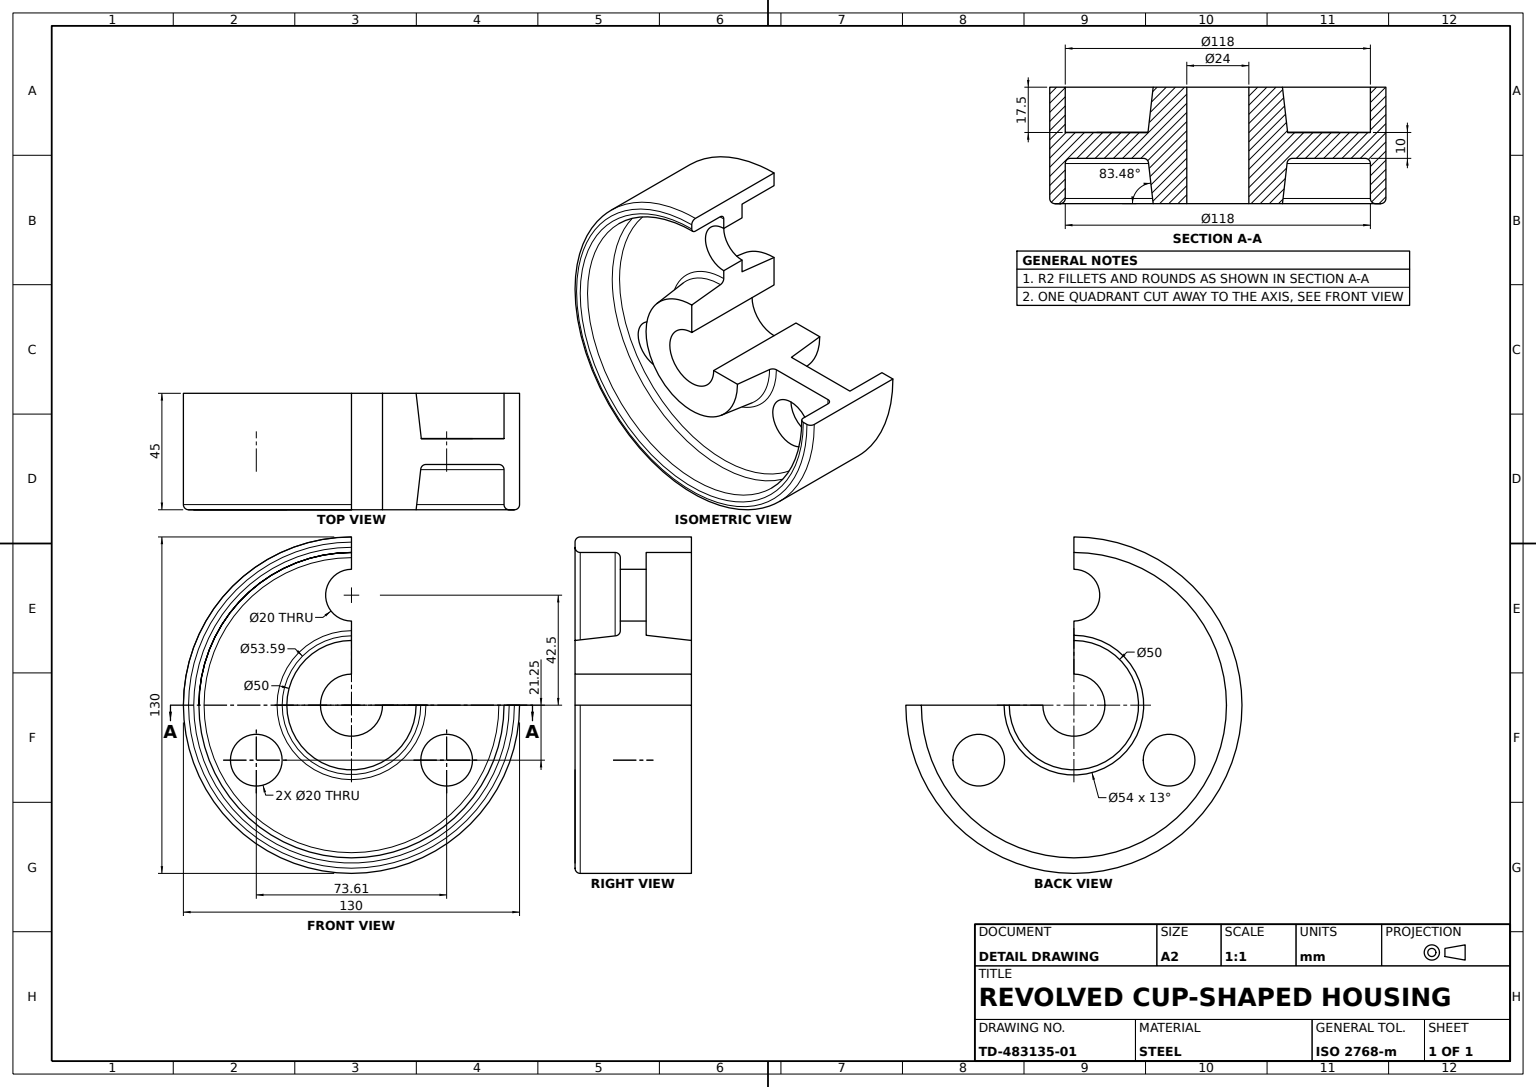
from build123d import *

# Parameters (mm, degrees)
RIM_SLOT_SKETCH_R         = 10
RIM_SLOT_CUT_DEPTH        = 96.949205312
EDGE_FILLET_R2_A_R        = 2
EDGE_FILLET_R2_B_R        = 2
WEB_RELIEF_CUT_DEPTH      = 96.94920538
WEB_RELIEF_CUT_DEPTH_BACK = 96.94920538


with BuildPart() as part:
    # Wheel Profile Sketch → Wheel Body Revolve (revolve)
    with BuildSketch(Plane.XY, mode=Mode.PRIVATE) as wheel_body_revolve_sk:
        Polygon((22.5, 12), (-22.5, 12), (-22.5, 25), (-5, 27), (-5, 59), (-22.5, 59), (-22.5, 65), (22.5, 65), (22.5, 59), (5, 59), (5, 27), (22.5, 25), align=None)
    revolve(wheel_body_revolve_sk.sketch.rotate(Axis((-53.084730572, 0, 0), (1, 0, 0)), 90), axis=Axis((-53.084730572, 0, 0), (1, 0, 0)))

    # Rim Slot Sketch → Rim Slot Cut (cut, through all)
    with BuildSketch(Plane(origin=(5, 0, 0), x_dir=(0, 0, -1), z_dir=(1, 0, 0))):
        with Locations((0, 42.5)):
            Circle(RIM_SLOT_SKETCH_R)
        with Locations((36.806079661, -21.25)):
            Circle(RIM_SLOT_SKETCH_R)
        with Locations((-36.806079661, -21.25)):
            Circle(RIM_SLOT_SKETCH_R)
    extrude(amount=-RIM_SLOT_CUT_DEPTH, mode=Mode.SUBTRACT)

    # Edge Fillet R2 A
    edge_fillet_r2_a_edges = [part.edges().sort_by_distance(p)[0] for p in [
        (22.5, 0, -65),
        (5, 0, -59),
        (5, 0, -27),
    ]]
    fillet(edge_fillet_r2_a_edges, radius=EDGE_FILLET_R2_A_R)

    # Edge Fillet R2 B
    edge_fillet_r2_b_edges = [part.edges().sort_by_distance(p)[0] for p in [
        (22.5, 0, -59),
    ]]
    fillet(edge_fillet_r2_b_edges, radius=EDGE_FILLET_R2_B_R)

    # Web Relief Sketch → Web Relief Cut (cut, two sides: drawn at the far end of the back side and taken through both)
    with BuildSketch(Plane(origin=(5, 0, 0), x_dir=(0, 0, -1), z_dir=(1, 0, 0)).offset(-WEB_RELIEF_CUT_DEPTH_BACK)):
        with BuildLine():
            Line((0, 77.992606611), (0, 0))
            Line((0, 0), (85.280618665, 0))
            ThreePointArc((85.280618665, 0), (62.367801888, 60.567229614), (0, 77.992606611))
        make_face()
    extrude(amount=WEB_RELIEF_CUT_DEPTH + WEB_RELIEF_CUT_DEPTH_BACK, mode=Mode.SUBTRACT)


solid = part.part
